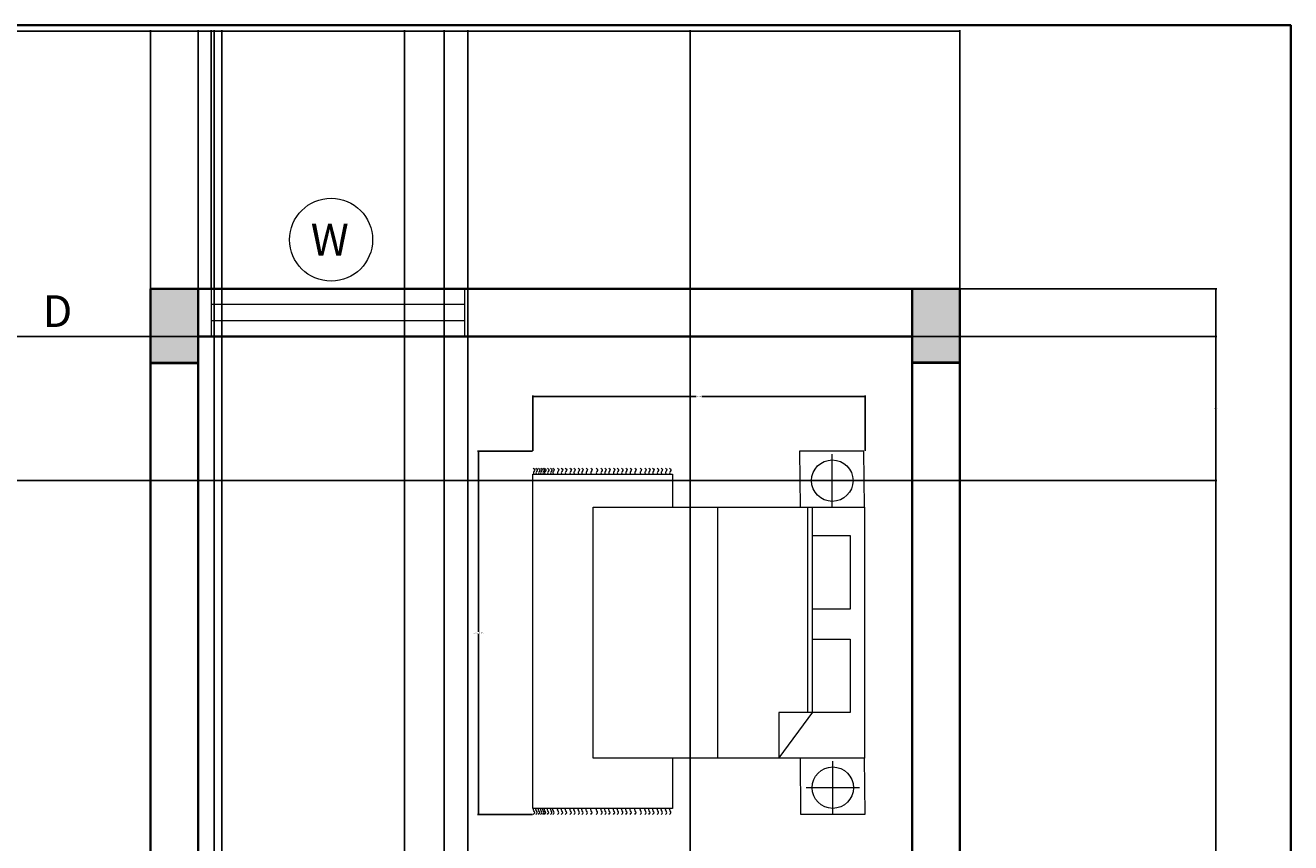
# Model space of a CAD drawing. Units: inches. Extents: x 2243 to 2668, y 14541 to 15226.
# Tile 5 of 5: x 2428 to 2668, y 15071 to 15226. Entities that reach past the tile are written whole.
import ezdxf

# ---------------------------------------------------------------- set-up
doc = ezdxf.new("R2010")
doc.units = ezdxf.units.IN
doc.header["$MEASUREMENT"] = 0
for name, color, linetype, lineweight in [('A-ANNO-DIMS', 2, 'Continuous', 18), ('A-ANNO-SYMB', 3, 'Continuous', 18), ('A-ANNO-TTLB', 7, 'Continuous', 35), ('A-COLS', 7, 'Continuous', 40), ('A-COLS-PATT', 7, 'Continuous', 13), ('A-FURN', 8, 'Continuous', 18), ('A-GLAZ', 4, 'Continuous', 18), ('A-WALL', 7, 'Continuous', 35)]:
    doc.layers.add(name, color=color, linetype=linetype, lineweight=lineweight)
doc.styles.get("Standard").update_dxf_attribs({"font": 'arial.ttf'})
doc.dimstyles.get("Standard").update_dxf_attribs({"dimtxt": 0.18, "dimasz": 0.18, "dimexe": 0.18, "dimexo": 0.0625, "dimgap": 0.09, "dimtad": 0, "dimtih": 1, "dimtoh": 1, "dimdec": 4, "dimzin": 0, "dimdsep": 46, "dimtxsty": 'Standard', "dimcen": 0.09, "dimadec": 0, "dimazin": 0, "dimtfac": 1, "dimtdec": 4, "dimtofl": 0, "dimtmove": 0, "dimatfit": 3, "dimfxl": 1, "dimtolj": 1, "dimtzin": 0, "dimarcsym": 0})

# ---------------------------------------------------------------- blocks, each defined once
blk = doc.blocks.new('BED-DOUBLE-WITH-NIGHTSTANDS')
for p, q in [((56.59, 58.08), (56.59, 68.14)), ((0, 64.36), (26.37, 64.36)), ((0, 1.12), (0, 64.36)), ((26.37, 64.36), (26.37, 58.06)), ((61.62, 63.11), (51.56, 63.11)), ((34.96, 10.66), (34.96, 58.08)), ((52, 19.27), (52, 58.08)), ((52.82, 19.32), (52.82, 58.08)), ((52.82, 19.32), (46.47, 10.71)), ((52.82, 19.27), (46.47, 19.27)), ((46.47, 19.27), (46.47, 10.71)), ((26.37, 10.66), (26.37, 1.12)), ((56.69, 0.03), (56.69, 10.09)), ((61.72, 5.06), (51.66, 5.06)), ((26.37, 1.12), (0, 1.12))]:
    blk.add_line(p, q)
for points in [[(50.39, 68.71), (50.5, 58.08), (62.68, 58.08), (62.58, 68.71)], [(62.68, 10.66), (11.36, 10.66), (11.36, 58.08), (62.68, 58.08)], [(59.98, 38.83), (52.82, 38.83), (52.82, 52.73), (59.98, 52.73)], [(59.98, 19.27), (52.82, 19.27), (52.82, 33.16), (59.98, 33.16)], [(50.5, 10.66), (50.6, 0.03), (62.78, 0.03), (62.68, 10.66)]]:
    blk.add_lwpolyline(points, close=True)
for centre in [(56.59, 63.11), (56.69, 5.06)]:
    blk.add_circle(centre, 3.92)
for points, knots in [([(0.07, 65.48), (0.19, 65.39), (0.43, 65.19), (0.19, 64.85), (0.02, 64.57), (0.13, 64.42), (0.18, 64.36)], [0, 0, 0, 0, 0.400747, 0.791423, 1.067667, 1.29709, 1.29709, 1.29709, 1.29709]), ([(0.57, 65.48), (0.7, 65.39), (0.94, 65.19), (0.7, 64.85), (0.52, 64.57), (0.63, 64.42), (0.68, 64.36)], [0, 0, 0, 0, 0.400747, 0.791423, 1.067667, 1.29709, 1.29709, 1.29709, 1.29709]), ([(1.06, 65.48), (1.18, 65.39), (1.42, 65.19), (1.18, 64.85), (1.01, 64.57), (1.11, 64.42), (1.16, 64.36)], [0, 0, 0, 0, 0.400747, 0.791423, 1.067667, 1.29709, 1.29709, 1.29709, 1.29709]), ([(1.46, 65.48), (1.58, 65.39), (1.82, 65.19), (1.58, 64.85), (1.4, 64.57), (1.51, 64.42), (1.56, 64.36)], [0, 0, 0, 0, 0.400747, 0.791423, 1.067667, 1.29709, 1.29709, 1.29709, 1.29709]), ([(1.88, 65.48), (2, 65.39), (2.24, 65.19), (2, 64.85), (1.82, 64.57), (1.93, 64.42), (1.98, 64.36)], [0, 0, 0, 0, 0.400747, 0.791423, 1.067667, 1.29709, 1.29709, 1.29709, 1.29709]), ([(2.18, 65.48), (2.31, 65.39), (2.55, 65.19), (2.31, 64.85), (2.13, 64.57), (2.24, 64.42), (2.29, 64.36)], [0, 0, 0, 0, 0.400747, 0.791423, 1.067667, 1.29709, 1.29709, 1.29709, 1.29709]), ([(2.76, 65.48), (2.88, 65.39), (3.12, 65.19), (2.88, 64.85), (2.71, 64.57), (2.81, 64.42), (2.86, 64.36)], [0, 0, 0, 0, 0.400747, 0.791423, 1.067667, 1.29709, 1.29709, 1.29709, 1.29709]), ([(3.32, 65.48), (3.45, 65.39), (3.7, 65.2), (3.44, 64.85), (3.27, 64.57), (3.38, 64.42), (3.43, 64.36)], [0, 0, 0, 0, 0.407265, 0.802015, 1.07826, 1.307683, 1.307683, 1.307683, 1.307683]), ([(3.75, 65.48), (3.88, 65.39), (4.11, 65.19), (3.88, 64.85), (3.7, 64.57), (3.81, 64.42), (3.86, 64.36)], [0, 0, 0, 0, 0.400747, 0.791423, 1.067667, 1.29709, 1.29709, 1.29709, 1.29709]), ([(4.64, 65.48), (4.76, 65.39), (5, 65.19), (4.76, 64.85), (4.58, 64.57), (4.69, 64.42), (4.74, 64.36)], [0, 0, 0, 0, 0.400747, 0.791423, 1.067667, 1.29709, 1.29709, 1.29709, 1.29709]), ([(5.36, 65.48), (5.49, 65.39), (5.73, 65.19), (5.49, 64.85), (5.31, 64.57), (5.42, 64.42), (5.47, 64.36)], [0, 0, 0, 0, 0.400747, 0.791423, 1.067667, 1.29709, 1.29709, 1.29709, 1.29709]), ([(6.12, 65.48), (6.24, 65.39), (6.48, 65.19), (6.24, 64.85), (6.07, 64.57), (6.17, 64.42), (6.22, 64.36)], [0, 0, 0, 0, 0.400747, 0.791423, 1.067667, 1.29709, 1.29709, 1.29709, 1.29709]), ([(7, 65.48), (7.12, 65.39), (7.36, 65.19), (7.12, 64.85), (6.95, 64.57), (7.05, 64.42), (7.1, 64.36)], [0, 0, 0, 0, 0.400747, 0.791423, 1.067667, 1.29709, 1.29709, 1.29709, 1.29709]), ([(7.73, 65.48), (7.85, 65.39), (8.09, 65.19), (7.85, 64.85), (7.68, 64.57), (7.78, 64.42), (7.83, 64.36)], [0, 0, 0, 0, 0.400747, 0.791423, 1.067667, 1.29709, 1.29709, 1.29709, 1.29709]), ([(8.54, 65.48), (8.66, 65.39), (8.9, 65.19), (8.66, 64.85), (8.49, 64.57), (8.6, 64.42), (8.65, 64.36)], [0, 0, 0, 0, 0.400747, 0.791423, 1.067667, 1.29709, 1.29709, 1.29709, 1.29709]), ([(9.23, 65.48), (9.35, 65.39), (9.59, 65.19), (9.35, 64.85), (9.18, 64.57), (9.29, 64.42), (9.34, 64.36)], [0, 0, 0, 0, 0.400747, 0.791423, 1.067667, 1.29709, 1.29709, 1.29709, 1.29709]), ([(10.05, 65.48), (10.17, 65.39), (10.41, 65.19), (10.17, 64.85), (10, 64.57), (10.1, 64.42), (10.15, 64.36)], [0, 0, 0, 0, 0.400747, 0.791423, 1.067667, 1.29709, 1.29709, 1.29709, 1.29709]), ([(10.93, 65.48), (11.05, 65.39), (11.29, 65.19), (11.05, 64.85), (10.88, 64.57), (10.99, 64.42), (11.03, 64.36)], [0, 0, 0, 0, 0.400747, 0.791423, 1.067667, 1.29709, 1.29709, 1.29709, 1.29709]), ([(11.97, 65.48), (12.09, 65.39), (12.33, 65.19), (12.09, 64.85), (11.92, 64.57), (12.02, 64.42), (12.07, 64.36)], [0, 0, 0, 0, 0.400747, 0.791423, 1.067667, 1.29709, 1.29709, 1.29709, 1.29709]), ([(12.85, 65.48), (12.97, 65.39), (13.21, 65.19), (12.97, 64.85), (12.8, 64.57), (12.9, 64.42), (12.95, 64.36)], [0, 0, 0, 0, 0.400747, 0.791423, 1.067667, 1.29709, 1.29709, 1.29709, 1.29709]), ([(13.58, 65.48), (13.7, 65.39), (13.94, 65.19), (13.7, 64.85), (13.53, 64.57), (13.63, 64.42), (13.68, 64.36)], [0, 0, 0, 0, 0.400747, 0.791423, 1.067667, 1.29709, 1.29709, 1.29709, 1.29709]), ([(14.33, 65.48), (14.45, 65.39), (14.69, 65.19), (14.45, 64.85), (14.28, 64.57), (14.38, 64.42), (14.43, 64.36)], [0, 0, 0, 0, 0.400747, 0.791423, 1.067667, 1.29709, 1.29709, 1.29709, 1.29709]), ([(15.21, 65.48), (15.33, 65.39), (15.57, 65.19), (15.33, 64.85), (15.16, 64.57), (15.27, 64.42), (15.32, 64.36)], [0, 0, 0, 0, 0.400747, 0.791423, 1.067667, 1.29709, 1.29709, 1.29709, 1.29709]), ([(15.94, 65.48), (16.06, 65.39), (16.3, 65.19), (16.06, 64.85), (15.89, 64.57), (15.99, 64.42), (16.04, 64.36)], [0, 0, 0, 0, 0.400747, 0.791423, 1.067667, 1.29709, 1.29709, 1.29709, 1.29709]), ([(16.76, 65.48), (16.88, 65.39), (17.12, 65.19), (16.88, 64.85), (16.7, 64.57), (16.81, 64.42), (16.86, 64.36)], [0, 0, 0, 0, 0.400747, 0.791423, 1.067667, 1.29709, 1.29709, 1.29709, 1.29709]), ([(17.53, 65.48), (17.65, 65.39), (17.89, 65.19), (17.65, 64.85), (17.48, 64.57), (17.59, 64.42), (17.64, 64.36)], [0, 0, 0, 0, 0.400747, 0.791423, 1.067667, 1.29709, 1.29709, 1.29709, 1.29709]), ([(18.35, 65.48), (18.47, 65.39), (18.71, 65.19), (18.47, 64.85), (18.3, 64.57), (18.4, 64.42), (18.45, 64.36)], [0, 0, 0, 0, 0.400747, 0.791423, 1.067667, 1.29709, 1.29709, 1.29709, 1.29709]), ([(19.23, 65.48), (19.35, 65.39), (19.59, 65.19), (19.35, 64.85), (19.18, 64.57), (19.29, 64.42), (19.33, 64.36)], [0, 0, 0, 0, 0.400747, 0.791423, 1.067667, 1.29709, 1.29709, 1.29709, 1.29709]), ([(20.27, 65.48), (20.39, 65.39), (20.63, 65.19), (20.39, 64.85), (20.22, 64.57), (20.32, 64.42), (20.37, 64.36)], [0, 0, 0, 0, 0.400747, 0.791423, 1.067667, 1.29709, 1.29709, 1.29709, 1.29709]), ([(21.15, 65.48), (21.27, 65.39), (21.51, 65.19), (21.27, 64.85), (21.1, 64.57), (21.21, 64.42), (21.25, 64.36)], [0, 0, 0, 0, 0.400747, 0.791423, 1.067667, 1.29709, 1.29709, 1.29709, 1.29709]), ([(21.88, 65.48), (22, 65.39), (22.24, 65.19), (22, 64.85), (21.83, 64.57), (21.93, 64.42), (21.98, 64.36)], [0, 0, 0, 0, 0.400747, 0.791423, 1.067667, 1.29709, 1.29709, 1.29709, 1.29709]), ([(22.63, 65.48), (22.75, 65.39), (22.99, 65.19), (22.75, 64.85), (22.58, 64.57), (22.69, 64.42), (22.73, 64.36)], [0, 0, 0, 0, 0.400747, 0.791423, 1.067667, 1.29709, 1.29709, 1.29709, 1.29709]), ([(23.51, 65.48), (23.63, 65.39), (23.87, 65.19), (23.63, 64.85), (23.46, 64.57), (23.57, 64.42), (23.62, 64.36)], [0, 0, 0, 0, 0.400747, 0.791423, 1.067667, 1.29709, 1.29709, 1.29709, 1.29709]), ([(24.24, 65.48), (24.36, 65.39), (24.6, 65.19), (24.36, 64.85), (24.19, 64.57), (24.3, 64.42), (24.34, 64.36)], [0, 0, 0, 0, 0.400747, 0.791423, 1.067667, 1.29709, 1.29709, 1.29709, 1.29709]), ([(25.06, 65.48), (25.18, 65.39), (25.42, 65.19), (25.18, 64.85), (25.01, 64.57), (25.11, 64.42), (25.16, 64.36)], [0, 0, 0, 0, 0.400747, 0.791423, 1.067667, 1.29709, 1.29709, 1.29709, 1.29709]), ([(25.84, 65.48), (25.96, 65.39), (26.2, 65.19), (25.96, 64.85), (25.78, 64.57), (25.89, 64.42), (25.94, 64.36)], [0, 0, 0, 0, 0.400747, 0.791423, 1.067667, 1.29709, 1.29709, 1.29709, 1.29709]), ([(0.07, 0), (0.19, 0.1), (0.43, 0.29), (0.19, 0.63), (0.02, 0.91), (0.13, 1.06), (0.18, 1.13)], [0, 0, 0, 0, 0.400747, 0.791423, 1.067667, 1.29709, 1.29709, 1.29709, 1.29709]), ([(0.55, 0), (0.67, 0.1), (0.91, 0.29), (0.67, 0.63), (0.49, 0.91), (0.6, 1.06), (0.65, 1.13)], [0, 0, 0, 0, 0.400747, 0.791423, 1.067667, 1.29709, 1.29709, 1.29709, 1.29709]), ([(1.03, 0), (1.15, 0.1), (1.39, 0.29), (1.15, 0.63), (0.98, 0.91), (1.09, 1.06), (1.13, 1.13)], [0, 0, 0, 0, 0.400747, 0.791423, 1.067667, 1.29709, 1.29709, 1.29709, 1.29709]), ([(1.43, 0), (1.55, 0.1), (1.79, 0.29), (1.55, 0.63), (1.38, 0.91), (1.48, 1.06), (1.53, 1.13)], [0, 0, 0, 0, 0.400747, 0.791423, 1.067667, 1.29709, 1.29709, 1.29709, 1.29709]), ([(1.85, 0), (1.97, 0.1), (2.21, 0.29), (1.97, 0.63), (1.8, 0.91), (1.9, 1.05), (1.94, 1.12)], [0, 0, 0, 0, 0.400747, 0.791423, 1.067667, 1.283686, 1.283686, 1.283686, 1.283686]), ([(2.16, 0), (2.28, 0.1), (2.52, 0.29), (2.28, 0.63), (2.11, 0.91), (2.21, 1.05), (2.25, 1.12)], [0, 0, 0, 0, 0.400747, 0.791423, 1.067667, 1.283686, 1.283686, 1.283686, 1.283686]), ([(2.73, 0), (2.85, 0.1), (3.09, 0.29), (2.85, 0.63), (2.68, 0.91), (2.78, 1.05), (2.82, 1.12)], [0, 0, 0, 0, 0.400747, 0.791423, 1.067667, 1.283686, 1.283686, 1.283686, 1.283686]), ([(3.32, 0), (3.45, 0.1), (3.69, 0.29), (3.45, 0.63), (3.27, 0.91), (3.38, 1.05), (3.42, 1.12)], [0, 0, 0, 0, 0.402903, 0.794912, 1.071156, 1.287177, 1.287177, 1.287177, 1.287177]), ([(3.75, 0), (3.88, 0.1), (4.11, 0.29), (3.88, 0.63), (3.7, 0.91), (3.8, 1.05), (3.85, 1.12)], [0, 0, 0, 0, 0.400747, 0.791423, 1.067667, 1.283686, 1.283686, 1.283686, 1.283686]), ([(4.64, 0), (4.76, 0.1), (5, 0.29), (4.76, 0.63), (4.59, 0.91), (4.69, 1.05), (4.73, 1.12)], [0, 0, 0, 0, 0.400747, 0.791423, 1.067667, 1.283686, 1.283686, 1.283686, 1.283686]), ([(5.36, 0), (5.49, 0.1), (5.73, 0.29), (5.49, 0.63), (5.31, 0.91), (5.42, 1.06), (5.47, 1.13)], [0, 0, 0, 0, 0.400747, 0.791423, 1.067667, 1.29709, 1.29709, 1.29709, 1.29709]), ([(6.12, 0), (6.24, 0.1), (6.48, 0.29), (6.24, 0.63), (6.07, 0.91), (6.17, 1.06), (6.22, 1.13)], [0, 0, 0, 0, 0.400747, 0.791423, 1.067667, 1.29709, 1.29709, 1.29709, 1.29709]), ([(7, 0), (7.12, 0.1), (7.36, 0.29), (7.12, 0.63), (6.95, 0.91), (7.05, 1.06), (7.1, 1.13)], [0, 0, 0, 0, 0.400747, 0.791423, 1.067667, 1.29709, 1.29709, 1.29709, 1.29709]), ([(7.73, 0), (7.85, 0.1), (8.09, 0.29), (7.85, 0.63), (7.68, 0.91), (7.78, 1.06), (7.83, 1.13)], [0, 0, 0, 0, 0.400747, 0.791423, 1.067667, 1.29709, 1.29709, 1.29709, 1.29709]), ([(8.54, 0), (8.66, 0.1), (8.9, 0.29), (8.66, 0.63), (8.49, 0.91), (8.6, 1.06), (8.65, 1.13)], [0, 0, 0, 0, 0.400747, 0.791423, 1.067667, 1.29709, 1.29709, 1.29709, 1.29709]), ([(9.23, 0), (9.35, 0.1), (9.59, 0.29), (9.35, 0.63), (9.18, 0.91), (9.29, 1.06), (9.34, 1.13)], [0, 0, 0, 0, 0.400747, 0.791423, 1.067667, 1.29709, 1.29709, 1.29709, 1.29709]), ([(10.05, 0), (10.17, 0.1), (10.41, 0.29), (10.17, 0.63), (10, 0.91), (10.1, 1.06), (10.15, 1.13)], [0, 0, 0, 0, 0.400747, 0.791423, 1.067667, 1.29709, 1.29709, 1.29709, 1.29709]), ([(10.93, 0), (11.05, 0.1), (11.29, 0.29), (11.05, 0.63), (10.88, 0.91), (10.99, 1.06), (11.03, 1.13)], [0, 0, 0, 0, 0.400747, 0.791423, 1.067667, 1.29709, 1.29709, 1.29709, 1.29709]), ([(11.97, 0), (12.09, 0.1), (12.33, 0.29), (12.09, 0.63), (11.92, 0.91), (12.02, 1.06), (12.07, 1.13)], [0, 0, 0, 0, 0.400747, 0.791423, 1.067667, 1.29709, 1.29709, 1.29709, 1.29709]), ([(12.85, 0), (12.97, 0.1), (13.21, 0.29), (12.97, 0.63), (12.8, 0.91), (12.9, 1.06), (12.95, 1.13)], [0, 0, 0, 0, 0.400747, 0.791423, 1.067667, 1.29709, 1.29709, 1.29709, 1.29709]), ([(13.58, 0), (13.7, 0.1), (13.94, 0.29), (13.7, 0.63), (13.53, 0.91), (13.63, 1.06), (13.68, 1.13)], [0, 0, 0, 0, 0.400747, 0.791423, 1.067667, 1.29709, 1.29709, 1.29709, 1.29709]), ([(14.33, 0), (14.45, 0.1), (14.69, 0.29), (14.45, 0.63), (14.28, 0.91), (14.38, 1.06), (14.43, 1.13)], [0, 0, 0, 0, 0.400747, 0.791423, 1.067667, 1.29709, 1.29709, 1.29709, 1.29709]), ([(15.21, 0), (15.33, 0.1), (15.57, 0.29), (15.33, 0.63), (15.16, 0.91), (15.27, 1.06), (15.32, 1.13)], [0, 0, 0, 0, 0.400747, 0.791423, 1.067667, 1.29709, 1.29709, 1.29709, 1.29709]), ([(15.94, 0), (16.06, 0.1), (16.3, 0.29), (16.06, 0.63), (15.89, 0.91), (15.99, 1.06), (16.04, 1.13)], [0, 0, 0, 0, 0.400747, 0.791423, 1.067667, 1.29709, 1.29709, 1.29709, 1.29709]), ([(16.76, 0), (16.88, 0.1), (17.12, 0.29), (16.88, 0.63), (16.7, 0.91), (16.81, 1.06), (16.86, 1.13)], [0, 0, 0, 0, 0.400747, 0.791423, 1.067667, 1.29709, 1.29709, 1.29709, 1.29709]), ([(17.53, 0), (17.65, 0.1), (17.89, 0.29), (17.65, 0.63), (17.48, 0.91), (17.59, 1.06), (17.64, 1.13)], [0, 0, 0, 0, 0.400747, 0.791423, 1.067667, 1.29709, 1.29709, 1.29709, 1.29709]), ([(18.35, 0), (18.47, 0.1), (18.71, 0.29), (18.47, 0.63), (18.3, 0.91), (18.4, 1.06), (18.45, 1.13)], [0, 0, 0, 0, 0.400747, 0.791423, 1.067667, 1.29709, 1.29709, 1.29709, 1.29709]), ([(19.23, 0), (19.35, 0.1), (19.59, 0.29), (19.35, 0.63), (19.18, 0.91), (19.29, 1.06), (19.33, 1.13)], [0, 0, 0, 0, 0.400747, 0.791423, 1.067667, 1.29709, 1.29709, 1.29709, 1.29709]), ([(20.27, 0), (20.39, 0.1), (20.63, 0.29), (20.39, 0.63), (20.22, 0.91), (20.32, 1.06), (20.37, 1.13)], [0, 0, 0, 0, 0.400747, 0.791423, 1.067667, 1.29709, 1.29709, 1.29709, 1.29709]), ([(21.15, 0), (21.27, 0.1), (21.51, 0.29), (21.27, 0.63), (21.1, 0.91), (21.21, 1.06), (21.25, 1.13)], [0, 0, 0, 0, 0.400747, 0.791423, 1.067667, 1.29709, 1.29709, 1.29709, 1.29709]), ([(21.88, 0), (22, 0.1), (22.24, 0.29), (22, 0.63), (21.83, 0.91), (21.93, 1.06), (21.98, 1.13)], [0, 0, 0, 0, 0.400747, 0.791423, 1.067667, 1.29709, 1.29709, 1.29709, 1.29709]), ([(22.63, 0), (22.75, 0.1), (22.99, 0.29), (22.75, 0.63), (22.58, 0.91), (22.69, 1.06), (22.73, 1.13)], [0, 0, 0, 0, 0.400747, 0.791423, 1.067667, 1.29709, 1.29709, 1.29709, 1.29709]), ([(23.51, 0), (23.63, 0.1), (23.87, 0.29), (23.63, 0.63), (23.46, 0.91), (23.57, 1.06), (23.62, 1.13)], [0, 0, 0, 0, 0.400747, 0.791423, 1.067667, 1.29709, 1.29709, 1.29709, 1.29709]), ([(24.24, 0), (24.36, 0.1), (24.6, 0.29), (24.36, 0.63), (24.19, 0.91), (24.3, 1.06), (24.34, 1.13)], [0, 0, 0, 0, 0.400747, 0.791423, 1.067667, 1.29709, 1.29709, 1.29709, 1.29709]), ([(25.06, 0), (25.18, 0.1), (25.42, 0.29), (25.18, 0.63), (25.01, 0.91), (25.11, 1.06), (25.16, 1.13)], [0, 0, 0, 0, 0.400747, 0.791423, 1.067667, 1.29709, 1.29709, 1.29709, 1.29709]), ([(25.84, 0), (25.96, 0.1), (26.2, 0.29), (25.96, 0.63), (25.78, 0.91), (25.89, 1.06), (25.94, 1.13)], [0, 0, 0, 0, 0.400747, 0.791423, 1.067667, 1.29709, 1.29709, 1.29709, 1.29709])]:
    blk.add_open_spline(points, degree=3, knots=knots)
blk = doc.blocks.new('WIN-48IN')
for p, q in [((0, 9), (0, 0)), ((48, 9), (0, 9)), ((48, 0), (48, 9)), ((48, 6), (0, 6)), ((0, 3), (48, 3)), ((0, 0), (48, 0))]:
    blk.add_line(p, q)
blk = doc.blocks.new('TAG-WINDOW-W')
blk.add_circle((7.84, 7.84), 7.84)
at = {"insert": (3.99, 10.84), "char_height": 6, "attachment_point": 1}
blk.add_mtext_dynamic_manual_height_columns('W', width=14.3449, gutter_width=30, heights=[0], dxfattribs=at)
blk = doc.blocks.new('*D11')
at = {"layer": 'A-ANNO-DIMS', "color": 0, "lineweight": -2, "transparency": 16777216}
for p, q in [((2524.2, 15145.46), (2513.78, 15145.46)), ((2513.96, 15145.28), (2513.96, 15111.29)), ((2513.96, 15076.93), (2513.96, 15110.92)), ((2524.2, 15076.75), (2513.78, 15076.75))]:
    blk.add_line(p, q, dxfattribs=at)
at = {"layer": 'A-ANNO-DIMS', "color": 0, "transparency": 16777216}
for points in [[(2513.93, 15145.28), (2513.99, 15145.28), (2513.96, 15145.46)], [(2513.93, 15076.93), (2513.99, 15076.93), (2513.96, 15076.75)]]:
    blk.add_solid(points, dxfattribs=at)
at = {"layer": 'Defpoints', "color": 0, "transparency": 16777216}
for p in [(2513.96, 15145.46), (2524.26, 15145.46), (2524.26, 15076.75)]:
    blk.add_point(p, dxfattribs=at)
at = {"layer": 'A-ANNO-DIMS', "color": 0, "transparency": 16777216, "insert": (2513.96, 15111.1), "char_height": 0.18, "attachment_point": 5}
blk.add_mtext('\\A1;BED SET 69 TYP.', dxfattribs=at)
blk = doc.blocks.new('*D12')
at = {"layer": 'A-ANNO-DIMS', "color": 0, "lineweight": -2, "transparency": 16777216}
for p, q in [((2524.26, 15145.52), (2524.26, 15155.94)), ((2587.05, 15145.52), (2587.05, 15155.94)), ((2524.44, 15155.76), (2555.13, 15155.76)), ((2586.87, 15155.76), (2556.18, 15155.76))]:
    blk.add_line(p, q, dxfattribs=at)
at = {"layer": 'A-ANNO-DIMS', "color": 0, "transparency": 16777216}
for points in [[(2524.44, 15155.79), (2524.44, 15155.73), (2524.26, 15155.76)], [(2586.87, 15155.79), (2586.87, 15155.73), (2587.05, 15155.76)]]:
    blk.add_solid(points, dxfattribs=at)
at = {"layer": 'Defpoints', "color": 0, "transparency": 16777216}
for p in [(2587.05, 15155.76), (2524.26, 15145.46), (2587.05, 15145.46)]:
    blk.add_point(p, dxfattribs=at)
at = {"layer": 'A-ANNO-DIMS', "color": 0, "transparency": 16777216, "insert": (2555.65, 15155.76), "char_height": 0.18, "attachment_point": 5}
blk.add_mtext('\\A1;63 TYP.', dxfattribs=at)
blk = doc.blocks.new('*D17')
at = {"layer": 'A-ANNO-DIMS', "color": 0, "lineweight": -2, "transparency": 16777216}
for p, q in [((2292.96, 15176.2), (2292.96, 15225.04)), ((2293.14, 15224.86), (2448.67, 15224.86)), ((2604.78, 15224.86), (2449.25, 15224.86)), ((2604.96, 15176.2), (2604.96, 15225.04))]:
    blk.add_line(p, q, dxfattribs=at)
at = {"layer": 'A-ANNO-DIMS', "color": 0, "transparency": 16777216}
for points in [[(2293.14, 15224.89), (2293.14, 15224.83), (2292.96, 15224.86)], [(2604.78, 15224.89), (2604.78, 15224.83), (2604.96, 15224.86)]]:
    blk.add_solid(points, dxfattribs=at)
at = {"layer": 'Defpoints', "color": 0, "transparency": 16777216}
for p in [(2604.96, 15224.86), (2292.96, 15176.14), (2604.96, 15176.14)]:
    blk.add_point(p, dxfattribs=at)
at = {"layer": 'A-ANNO-DIMS', "color": 0, "transparency": 16777216, "insert": (2448.96, 15224.86), "char_height": 0.18, "attachment_point": 5}
blk.add_mtext('\\A1;312', dxfattribs=at)
blk = doc.blocks.new('*D18')
at = {"layer": 'A-ANNO-DIMS', "color": 0, "lineweight": -2, "transparency": 16777216}
for p, q in [((2605.02, 15176.14), (2653.58, 15176.14)), ((2653.4, 15175.96), (2653.4, 14877.07)), ((2653.4, 14577.82), (2653.4, 14876.7)), ((2605.02, 14577.64), (2653.58, 14577.64))]:
    blk.add_line(p, q, dxfattribs=at)
at = {"layer": 'A-ANNO-DIMS', "color": 0, "transparency": 16777216}
for points in [[(2653.37, 15175.96), (2653.43, 15175.96), (2653.4, 15176.14)], [(2653.37, 14577.82), (2653.43, 14577.82), (2653.4, 14577.64)]]:
    blk.add_solid(points, dxfattribs=at)
at = {"layer": 'Defpoints', "color": 0, "transparency": 16777216}
for p in [(2604.96, 15176.14), (2653.4, 15176.14), (2604.96, 14577.64)]:
    blk.add_point(p, dxfattribs=at)
at = {"layer": 'A-ANNO-DIMS', "color": 0, "transparency": 16777216, "insert": (2653.4, 14876.89), "char_height": 0.18, "attachment_point": 5}
blk.add_mtext('\\A1;598.5', dxfattribs=at)
blk = doc.blocks.new('*D35')
at = {"layer": 'A-ANNO-DIMS', "color": 0, "lineweight": -2, "transparency": 16777216}
for p, q in [((2411.89, 14673.7), (2411.89, 15225.04)), ((2412.07, 15224.86), (2431.53, 15224.86)), ((2451.78, 15224.86), (2432.32, 15224.86)), ((2451.96, 14673.7), (2451.96, 15225.04))]:
    blk.add_line(p, q, dxfattribs=at)
at = {"layer": 'A-ANNO-DIMS', "color": 0, "transparency": 16777216}
for points in [[(2412.07, 15224.89), (2412.07, 15224.83), (2411.89, 15224.86)], [(2451.78, 15224.89), (2451.78, 15224.83), (2451.96, 15224.86)]]:
    blk.add_solid(points, dxfattribs=at)
at = {"layer": 'Defpoints', "color": 0, "transparency": 16777216}
for p in [(2451.96, 15224.86), (2411.89, 14673.64), (2451.96, 14673.64)]:
    blk.add_point(p, dxfattribs=at)
at = {"layer": 'A-ANNO-DIMS', "color": 0, "transparency": 16777216, "insert": (2431.93, 15224.86), "char_height": 0.18, "attachment_point": 5}
blk.add_mtext('\\A1;40.07', dxfattribs=at)
blk = doc.blocks.new('*D36')
at = {"layer": 'A-ANNO-DIMS', "color": 0, "lineweight": -2, "transparency": 16777216}
for p, q in [((2460.96, 14673.7), (2460.96, 15225.04)), ((2461.14, 15224.86), (2462.95, 15224.86)), ((2465.28, 15224.86), (2463.47, 15224.86)), ((2465.46, 14673.7), (2465.46, 15225.04))]:
    blk.add_line(p, q, dxfattribs=at)
at = {"layer": 'A-ANNO-DIMS', "color": 0, "transparency": 16777216}
for points in [[(2461.14, 15224.89), (2461.14, 15224.83), (2460.96, 15224.86)], [(2465.28, 15224.89), (2465.28, 15224.83), (2465.46, 15224.86)]]:
    blk.add_solid(points, dxfattribs=at)
at = {"layer": 'Defpoints', "color": 0, "transparency": 16777216}
for p in [(2465.46, 15224.86), (2460.96, 14673.64), (2465.46, 14673.64)]:
    blk.add_point(p, dxfattribs=at)
at = {"layer": 'A-ANNO-DIMS', "color": 0, "transparency": 16777216, "insert": (2463.21, 15224.86), "char_height": 0.18, "attachment_point": 5}
blk.add_mtext('\\A1;4.5', dxfattribs=at)
blk = doc.blocks.new('*D37')
at = {"layer": 'A-ANNO-DIMS', "color": 0, "lineweight": -2, "transparency": 16777216}
for p, q in [((2463.96, 14586.7), (2463.96, 15225.04)), ((2464.14, 15224.86), (2508.74, 15224.86)), ((2553.78, 15224.86), (2509.18, 15224.86)), ((2553.96, 14586.7), (2553.96, 15225.04))]:
    blk.add_line(p, q, dxfattribs=at)
at = {"layer": 'A-ANNO-DIMS', "color": 0, "transparency": 16777216}
for points in [[(2464.14, 15224.89), (2464.14, 15224.83), (2463.96, 15224.86)], [(2553.78, 15224.89), (2553.78, 15224.83), (2553.96, 15224.86)]]:
    blk.add_solid(points, dxfattribs=at)
at = {"layer": 'Defpoints', "color": 0, "transparency": 16777216}
for p in [(2553.96, 15224.86), (2463.96, 14586.64), (2553.96, 14586.64)]:
    blk.add_point(p, dxfattribs=at)
at = {"layer": 'A-ANNO-DIMS', "color": 0, "transparency": 16777216, "insert": (2508.96, 15224.86), "char_height": 0.18, "attachment_point": 5}
blk.add_mtext('\\A1;90', dxfattribs=at)
blk = doc.blocks.new('*D40')
at = {"layer": 'A-ANNO-DIMS', "color": 0, "lineweight": -2, "transparency": 16777216}
for p, q in [((2451.96, 15176.2), (2451.96, 15225.04)), ((2452.14, 15224.86), (2457.29, 15224.86)), ((2463.21, 15224.86), (2458.06, 15224.86)), ((2463.39, 15176.2), (2463.39, 15225.04))]:
    blk.add_line(p, q, dxfattribs=at)
at = {"layer": 'A-ANNO-DIMS', "color": 0, "transparency": 16777216}
for points in [[(2452.14, 15224.89), (2452.14, 15224.83), (2451.96, 15224.86)], [(2463.21, 15224.89), (2463.21, 15224.83), (2463.39, 15224.86)]]:
    blk.add_solid(points, dxfattribs=at)
at = {"layer": 'Defpoints', "color": 0, "transparency": 16777216}
for p in [(2463.39, 15224.86), (2451.96, 15176.14), (2463.39, 15176.14)]:
    blk.add_point(p, dxfattribs=at)
at = {"layer": 'A-ANNO-DIMS', "color": 0, "transparency": 16777216, "insert": (2457.68, 15224.86), "char_height": 0.18, "attachment_point": 5}
blk.add_mtext('\\A1;11.43', dxfattribs=at)
blk = doc.blocks.new('*D41')
at = {"layer": 'A-ANNO-DIMS', "color": 0, "lineweight": -2, "transparency": 16777216}
for p, q in [((2415.96, 15176.2), (2415.96, 15225.04)), ((2416.14, 15224.86), (2433.74, 15224.86)), ((2451.78, 15224.86), (2434.18, 15224.86)), ((2451.96, 15176.2), (2451.96, 15225.04))]:
    blk.add_line(p, q, dxfattribs=at)
at = {"layer": 'A-ANNO-DIMS', "color": 0, "transparency": 16777216}
for points in [[(2416.14, 15224.89), (2416.14, 15224.83), (2415.96, 15224.86)], [(2451.78, 15224.89), (2451.78, 15224.83), (2451.96, 15224.86)]]:
    blk.add_solid(points, dxfattribs=at)
at = {"layer": 'Defpoints', "color": 0, "transparency": 16777216}
for p in [(2451.96, 15224.86), (2415.96, 15176.14), (2451.96, 15176.14)]:
    blk.add_point(p, dxfattribs=at)
at = {"layer": 'A-ANNO-DIMS', "color": 0, "transparency": 16777216, "insert": (2433.96, 15224.86), "char_height": 0.18, "attachment_point": 5}
blk.add_mtext('\\A1;36', dxfattribs=at)
blk = doc.blocks.new('*D44')
at = {"layer": 'A-ANNO-DIMS', "color": 0, "lineweight": -2, "transparency": 16777216}
for p, q in [((2302.02, 15167.14), (2653.58, 15167.14)), ((2653.4, 15166.96), (2653.4, 15153.7)), ((2653.4, 15140.08), (2653.4, 15153.34)), ((2334.52, 15139.9), (2653.58, 15139.9))]:
    blk.add_line(p, q, dxfattribs=at)
at = {"layer": 'A-ANNO-DIMS', "color": 0, "transparency": 16777216}
for points in [[(2653.37, 15166.96), (2653.43, 15166.96), (2653.4, 15167.14)], [(2653.37, 15140.08), (2653.43, 15140.08), (2653.4, 15139.9)]]:
    blk.add_solid(points, dxfattribs=at)
at = {"layer": 'Defpoints', "color": 0, "transparency": 16777216}
for p in [(2301.96, 15167.14), (2653.4, 15167.14), (2334.46, 15139.9)]:
    blk.add_point(p, dxfattribs=at)
at = {"layer": 'A-ANNO-DIMS', "color": 0, "transparency": 16777216, "insert": (2653.4, 15153.52), "char_height": 0.18, "attachment_point": 5}
blk.add_mtext('\\A1;27.24', dxfattribs=at)
blk = doc.blocks.new('*D48')
at = {"layer": 'A-ANNO-DIMS', "color": 0, "lineweight": -2, "transparency": 16777216}
for p, q in [((2463.96, 14891.2), (2463.96, 15225.04)), ((2464.14, 15224.86), (2481.74, 15224.86)), ((2499.78, 15224.86), (2482.18, 15224.86)), ((2499.96, 14891.2), (2499.96, 15225.04))]:
    blk.add_line(p, q, dxfattribs=at)
at = {"layer": 'A-ANNO-DIMS', "color": 0, "transparency": 16777216}
for points in [[(2464.14, 15224.89), (2464.14, 15224.83), (2463.96, 15224.86)], [(2499.78, 15224.89), (2499.78, 15224.83), (2499.96, 15224.86)]]:
    blk.add_solid(points, dxfattribs=at)
at = {"layer": 'Defpoints', "color": 0, "transparency": 16777216}
for p in [(2499.96, 15224.86), (2463.96, 14891.14), (2499.96, 14891.14)]:
    blk.add_point(p, dxfattribs=at)
at = {"layer": 'A-ANNO-DIMS', "color": 0, "transparency": 16777216, "insert": (2481.96, 15224.86), "char_height": 0.18, "attachment_point": 5}
blk.add_mtext('\\A1;36', dxfattribs=at)
blk = doc.blocks.new('*D52')
at = {"layer": 'A-ANNO-DIMS', "color": 0, "lineweight": -2, "transparency": 16777216}
for p, q in [((2460.96, 15014.2), (2460.96, 15225.04)), ((2461.14, 15224.86), (2483.88, 15224.86)), ((2507.28, 15224.86), (2484.54, 15224.86)), ((2507.46, 15023.2), (2507.46, 15225.04))]:
    blk.add_line(p, q, dxfattribs=at)
at = {"layer": 'A-ANNO-DIMS', "color": 0, "transparency": 16777216}
for points in [[(2461.14, 15224.89), (2461.14, 15224.83), (2460.96, 15224.86)], [(2507.28, 15224.89), (2507.28, 15224.83), (2507.46, 15224.86)]]:
    blk.add_solid(points, dxfattribs=at)
at = {"layer": 'Defpoints', "color": 0, "transparency": 16777216}
for p in [(2507.46, 15224.86), (2507.46, 15023.14), (2460.96, 15014.14)]:
    blk.add_point(p, dxfattribs=at)
at = {"layer": 'A-ANNO-DIMS', "color": 0, "transparency": 16777216, "insert": (2484.21, 15224.86), "char_height": 0.18, "attachment_point": 5}
blk.add_mtext('\\A1;46.5', dxfattribs=at)
blk = doc.blocks.new('*D55')
at = {"layer": 'A-ANNO-DIMS', "color": 0, "lineweight": -2, "transparency": 16777216}
for p, q in [((2507.46, 14970.7), (2507.46, 15225.04)), ((2507.64, 15224.86), (2509.45, 15224.86)), ((2511.78, 15224.86), (2509.97, 15224.86)), ((2511.96, 14970.7), (2511.96, 15225.04))]:
    blk.add_line(p, q, dxfattribs=at)
at = {"layer": 'A-ANNO-DIMS', "color": 0, "transparency": 16777216}
for points in [[(2507.64, 15224.89), (2507.64, 15224.83), (2507.46, 15224.86)], [(2511.78, 15224.89), (2511.78, 15224.83), (2511.96, 15224.86)]]:
    blk.add_solid(points, dxfattribs=at)
at = {"layer": 'Defpoints', "color": 0, "transparency": 16777216}
for p in [(2507.46, 15224.86), (2507.46, 14970.64), (2511.96, 14970.64)]:
    blk.add_point(p, dxfattribs=at)
at = {"layer": 'A-ANNO-DIMS', "color": 0, "transparency": 16777216, "insert": (2509.71, 15224.86), "char_height": 0.18, "attachment_point": 5}
blk.add_mtext('\\A1;4.5', dxfattribs=at)

msp = doc.modelspace()

# ---------------------------------------------------------------- hatches: boundary and pattern name
at = {"layer": 'A-COLS-PATT'}
h = msp.add_hatch(color=256, dxfattribs=at)
h.dxf.hatch_style = 1
h.paths.add_polyline_path([(2301.96, 15176.1368), (2292.96, 15176.1368), (2292.96, 15162.1368), (2301.96, 15162.1368)])
h.paths.add_polyline_path([(2460.96, 15176.1368), (2451.96, 15176.1368), (2451.96, 15162.1368), (2460.96, 15162.1368)])
h.paths.add_polyline_path([(2604.96, 15176.1368), (2595.96, 15176.1368), (2595.96, 15162.1368), (2604.96, 15162.1368)])
h.paths.add_polyline_path([(2301.96, 15028.1368), (2292.96, 15028.1368), (2292.96, 15014.1368), (2301.96, 15014.1368)])
h.paths.add_polyline_path([(2460.96, 15028.1368), (2451.96, 15028.1368), (2451.96, 15014.1368), (2460.96, 15014.1368)])
h.paths.add_polyline_path([(2604.96, 15027.8868), (2595.96, 15027.8868), (2595.96, 15013.8868), (2604.96, 15013.8868)])
h.paths.add_polyline_path([(2301.96, 14891.1368), (2292.96, 14891.1368), (2292.96, 14877.1368), (2301.96, 14877.1368)])
h.paths.add_polyline_path([(2460.96, 14891.1368), (2451.96, 14891.1368), (2451.96, 14877.1368), (2460.96, 14877.1368)])
h.paths.add_polyline_path([(2604.96, 14891.1368), (2595.96, 14891.1368), (2595.96, 14877.1368), (2604.96, 14877.1368)])
h.paths.add_polyline_path([(2301.96, 14678.6368), (2292.96, 14678.6368), (2292.96, 14664.6368), (2301.96, 14664.6368)])
h.paths.add_polyline_path([(2460.96, 14678.6368), (2451.96, 14678.6368), (2451.96, 14664.6368), (2460.96, 14664.6368)])
h.paths.add_polyline_path([(2604.96, 14678.6368), (2595.96, 14678.6368), (2595.96, 14664.6368), (2604.96, 14664.6368)])
h.paths.add_polyline_path([(2604.96, 14591.6368), (2595.96, 14591.6368), (2595.96, 14577.6368), (2604.96, 14577.6368)])
h.paths.add_polyline_path([(2460.96, 14591.6368), (2451.96, 14591.6368), (2451.96, 14577.6368), (2460.96, 14577.6368)])
h.paths.add_polyline_path([(2306.96, 14586.6368), (2292.96, 14586.6368), (2292.96, 14577.6368), (2306.96, 14577.6368)])

# ---------------------------------------------------------------- linework, layer by layer
at = {"layer": 'A-ANNO-TTLB'}
msp.add_lwpolyline([(2246.1122, 15225.9536), (2667.5226, 15225.9536), (2667.5226, 14540.814), (2246.1122, 14540.814)], close=True, dxfattribs=at)
at = {"layer": 'A-COLS'}
for p, q in [((2451.96, 15162.1368), (2460.96, 15162.1368)), ((2604.96, 15162.1368), (2595.96, 15162.1368))]:
    msp.add_line(p, q, dxfattribs=at)
at = {"layer": 'A-WALL'}
for p, q in [((2451.96, 15176.1368), (2451.96, 15014.1368)), ((2451.96, 15176.1368), (2604.96, 15176.1368)), ((2460.96, 15176.1368), (2460.96, 15014.1368)), ((2595.96, 15176.1368), (2595.96, 14970.6368)), ((2604.96, 15176.1368), (2604.96, 14577.6368)), ((2460.96, 15167.1368), (2595.96, 15167.1368))]:
    msp.add_line(p, q, dxfattribs=at)

# ---------------------------------------------------------------- block references
at = {"layer": 'A-ANNO-SYMB'}
msp.add_blockref('TAG-WINDOW-W', (2478.259, 15177.577), dxfattribs=at)
at = {"layer": 'A-FURN'}
msp.add_blockref('BED-DOUBLE-WITH-NIGHTSTANDS', (2524.262, 15076.748), dxfattribs=at)
at = {"layer": 'A-GLAZ'}
msp.add_blockref('WIN-48IN', (2463.391, 15167.137), dxfattribs=at)

# ---------------------------------------------------------------- texts
at = {"layer": 'A-ANNO-SYMB', "insert": (2431.5354, 15174.9055), "char_height": 6, "attachment_point": 1}
msp.add_mtext_dynamic_manual_height_columns('D', width=14.74723, gutter_width=30, heights=[0], dxfattribs=at)

# ---------------------------------------------------------------- dimensions: what is measured, and where the dimension line sits
at = {"layer": 'A-ANNO-DIMS'}
for base, p1, p2, override, picture, middle in [((2604.96, 15224.8619), (2292.96, 15176.1368), (2604.96, 15176.1368), {"dimdec": 0, "dimlfac": 1, "dimrnd": 0, "dimzin": 0, "dimdsep": 46, "dimlunit": 2}, '*D17', (2448.96, 15224.8619)), ((2451.96, 15224.8619), (2411.8914, 14673.6368), (2451.96, 14673.6368), {"dimdec": 2, "dimlfac": 1, "dimrnd": 0, "dimzin": 0, "dimdsep": 46, "dimlunit": 2}, '*D35', (2431.9257, 15224.8619)), ((2451.96, 15224.8619), (2415.96, 15176.1368), (2451.96, 15176.1368), {"dimdec": 0, "dimlfac": 1, "dimrnd": 0, "dimzin": 0, "dimdsep": 46, "dimlunit": 2}, '*D41', (2433.96, 15224.8619)), ((2463.391, 15224.8619), (2451.96, 15176.1368), (2463.391, 15176.1368), {"dimdec": 2, "dimlfac": 1, "dimrnd": 0, "dimzin": 0, "dimdsep": 46, "dimlunit": 2}, '*D40', (2457.6755, 15224.8619)), ((2465.46, 15224.8619), (2460.96, 14673.6368), (2465.46, 14673.6368), {"dimdec": 1, "dimlfac": 1, "dimrnd": 0, "dimzin": 0, "dimdsep": 46, "dimlunit": 2}, '*D36', (2463.21, 15224.8619)), ((2507.46, 15224.8619), (2460.96, 15014.1368), (2507.46, 15023.1368), {"dimdec": 1, "dimlfac": 1, "dimrnd": 0, "dimzin": 0, "dimdsep": 46, "dimlunit": 2}, '*D52', (2484.21, 15224.8619)), ((2553.96, 15224.8619), (2463.96, 14586.6368), (2553.96, 14586.6368), {"dimdec": 0, "dimlfac": 1, "dimrnd": 0, "dimzin": 0, "dimdsep": 46, "dimlunit": 2}, '*D37', (2508.96, 15224.8619)), ((2499.96, 15224.8619), (2463.96, 14891.1368), (2499.96, 14891.1368), {"dimdec": 0, "dimlfac": 1, "dimrnd": 0, "dimzin": 0, "dimdsep": 46, "dimlunit": 2}, '*D48', (2481.96, 15224.8619)), ((2507.46, 15224.8619), (2511.96, 14970.6368), (2507.46, 14970.6368), {"dimdec": 1, "dimlfac": 1, "dimrnd": 0, "dimzin": 0, "dimdsep": 46, "dimlunit": 2}, '*D55', (2509.71, 15224.8619))]:
    dim = msp.add_linear_dim(base=base, p1=p1, p2=p2, dimstyle='Standard', override=override, dxfattribs=at)
    dim.commit()
    dim.dimension.update_dxf_attribs({"geometry": picture, "text_midpoint": middle})
for base, p1, p2, override, picture, middle in [((2653.4036, 15176.1368), (2604.96, 14577.6368), (2604.96, 15176.1368), {"dimdec": 1, "dimlfac": 1, "dimrnd": 0, "dimzin": 0, "dimdsep": 46, "dimlunit": 2}, '*D18', (2653.4036, 14876.8868)), ((2653.4036, 15167.1368), (2334.4616, 15139.8973), (2301.96, 15167.1368), {"dimdec": 2, "dimlfac": 1, "dimrnd": 0, "dimzin": 0, "dimdsep": 46, "dimlunit": 2}, '*D44', (2653.4036, 15153.5171))]:
    dim = msp.add_linear_dim(base=base, p1=p1, p2=p2, angle=90, dimstyle='Standard', override=override, dxfattribs=at)
    dim.commit()
    dim.dimension.update_dxf_attribs({"geometry": picture, "text_midpoint": middle})
dim = msp.add_linear_dim(base=(2587.0455, 15155.7646), p1=(2524.262, 15145.4581), p2=(2587.0455, 15145.4581), text='<> TYP.', dimstyle='Standard', override={"dimdec": 0, "dimlfac": 1, "dimrnd": 0, "dimzin": 0, "dimdsep": 46, "dimlunit": 2}, dxfattribs=at)
dim.commit()
dim.dimension.update_dxf_attribs({"geometry": '*D12', "text_midpoint": (2555.6538, 15155.7646)})
dim = msp.add_linear_dim(base=(2513.9555, 15145.4581), p1=(2524.262, 15076.7482), p2=(2524.262, 15145.4581), angle=90, text='BED SET <> TYP.', dimstyle='Standard', override={"dimdec": 0, "dimlfac": 1, "dimrnd": 0, "dimzin": 0, "dimdsep": 46, "dimlunit": 2}, dxfattribs=at)
dim.commit()
dim.dimension.update_dxf_attribs({"geometry": '*D11', "text_midpoint": (2513.9555, 15111.1031)})

doc.saveas('drawing.dxf')
